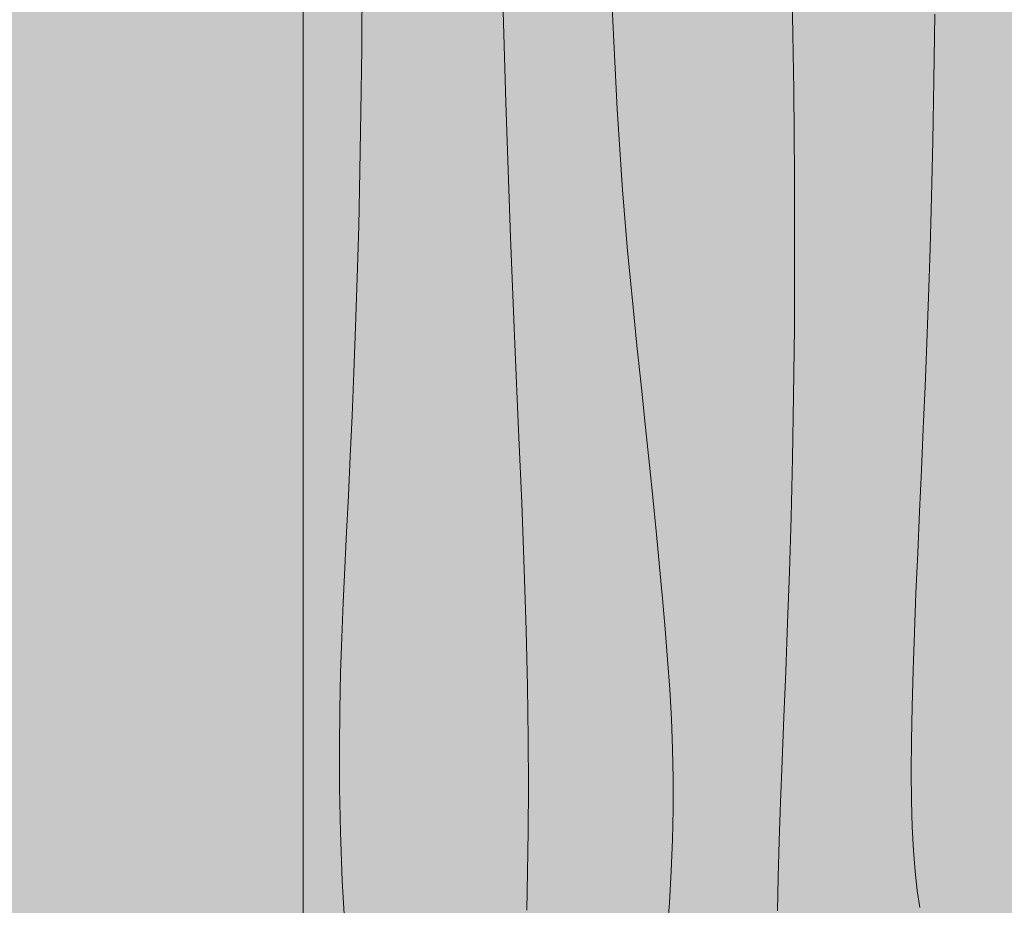
# Model space of a CAD drawing. Units: inches. Extents: x 3024 to 3952, y 1308 to 1863.
# Tile 15 of 29: x 3391.52 to 3411.08, y 1506.34 to 1523.92. Entities that reach past the tile are written whole.
import ezdxf

# ---------------------------------------------------------------- set-up
doc = ezdxf.new("R2010")
doc.units = ezdxf.units.IN
for name, color, linetype, lineweight in [('A-ANNO-DIMS', 2, 'Continuous', 18), ('A-FLOR-TILE-PATT', 7, 'Continuous', 13), ('A-FURN', 8, 'Continuous', 18), ('A-FURN-PATT', 9, 'Continuous', 13)]:
    doc.layers.add(name, color=color, linetype=linetype, lineweight=lineweight)
doc.layers.add('A-FLOR-PATT', color=254, linetype='Continuous', lineweight=13, true_color=0xfeeab9)
doc.styles.get("Standard").update_dxf_attribs({"font": 'arial.ttf'})
doc.dimstyles.get("Standard").update_dxf_attribs({"dimtxt": 0.18, "dimasz": 0.18, "dimexe": 0.18, "dimexo": 0.0625, "dimgap": 0.09, "dimtad": 0, "dimtih": 1, "dimtoh": 1, "dimdec": 4, "dimzin": 0, "dimdsep": 46, "dimtxsty": 'Standard', "dimcen": 0.09, "dimadec": 0, "dimazin": 0, "dimtfac": 1, "dimtdec": 4, "dimtofl": 0, "dimtmove": 0, "dimatfit": 3, "dimfxl": 1, "dimtolj": 1, "dimtzin": 0, "dimarcsym": 0})

# ---------------------------------------------------------------- blocks, each defined once
blk = doc.blocks.new('Table - Rectangular Woodgrain 60 x 30 in.')
blk.add_line((0, -30), (60, -30))
for points in [[(23.6054, -13.2439), (25.3666, -13.2667), (26.9728, -13.2947), (28.4531, -13.3281), (29.8256, -13.3663), (31.1083, -13.4083), (32.3191, -13.4535), (33.476, -13.501), (34.597, -13.5501), (35.7, -13.6), (36.7984, -13.6497), (37.8875, -13.6979), (38.9578, -13.743), (40, -13.7833), (41.0047, -13.8174), (41.9625, -13.8438), (42.864, -13.8607), (43.7, -13.8667), (44.4631, -13.8604), (45.1552, -13.8417), (45.7801, -13.8104), (46.3416, -13.7667), (46.8439, -13.7104), (47.2906, -13.6417)], [(23.1328, -17.0297), (25.6307, -16.9878), (27.9, -16.9667), (29.9928, -16.9617), (31.9302, -16.9703), (33.7254, -16.9907), (35.3917, -17.0208), (36.9423, -17.0588), (38.3906, -17.1026), (39.7499, -17.1503), (41.0333, -17.2), (42.2519, -17.2496), (43.4073, -17.2969), (44.4986, -17.3395), (45.525, -17.375), (46.4858, -17.4012), (47.3802, -17.4156)], [(23.25, -21.8083), (26.1269, -21.6663), (28.2656, -21.5281), (29.884, -21.3947), (31.2, -21.2667), (32.3967, -21.1448), (33.5172, -21.0292), (34.5697, -20.9198), (35.5625, -20.8167), (36.5037, -20.7198), (37.4015, -20.6292), (38.2642, -20.5448), (39.1, -20.4667), (39.9164, -20.3951), (40.7187, -20.3313), (41.5117, -20.2768), (42.3, -20.2333), (43.0883, -20.2024), (43.8812, -20.1854), (44.6836, -20.1841), (45.5, -20.2), (46.3328, -20.234), (47.1747, -20.2844), (48.0163, -20.3488)], [(21.4049, -24.7606), (25.9458, -24.625), (29.529, -24.4988), (32.3578, -24.3844), (34.6359, -24.284), (36.5667, -24.2), (38.3213, -24.1341), (39.9417, -24.0854), (41.437, -24.0523), (42.8167, -24.0333), (44.0901, -24.0268), (45.2667, -24.0313), (46.3557, -24.0451), (47.3667, -24.0667)], [(22.6125, -28.4344), (24.5164, -28.4455), (26.2, -28.4667), (27.762, -28.4947), (29.2276, -28.5281), (30.6033, -28.5663), (31.8958, -28.6084), (33.1118, -28.6535), (34.2578, -28.7011), (35.3405, -28.7501), (36.3666, -28.8), (37.3443, -28.8497), (38.288, -28.8974), (39.2137, -28.9412), (40.1375, -28.9792), (41.0753, -29.0093), (42.0432, -29.0297), (43.0572, -29.0384), (44.1333, -29.0333), (45.2936, -29.0114), (46.5843, -28.9641), (48.0579, -28.8816)]]:
    blk.add_lwpolyline(points)
blk = doc.blocks.new('*D32')
at = {"layer": 'A-ANNO-DIMS', "color": 0, "lineweight": -2, "transparency": 16777216}
for p, q in [((3397.088, 1541.715), (3390.23, 1541.715)), ((3390.41, 1541.535), (3390.41, 1519.428)), ((3390.41, 1496.958), (3390.41, 1519.065)), ((3397.088, 1496.778), (3390.23, 1496.778))]:
    blk.add_line(p, q, dxfattribs=at)
at = {"layer": 'A-ANNO-DIMS', "color": 0, "transparency": 16777216}
for points in [[(3390.38, 1541.535), (3390.44, 1541.535), (3390.41, 1541.715)], [(3390.38, 1496.958), (3390.44, 1496.958), (3390.41, 1496.778)]]:
    blk.add_solid(points, dxfattribs=at)
at = {"layer": 'Defpoints', "color": 0, "transparency": 16777216}
for p in [(3397.15, 1541.715), (3390.41, 1496.778), (3397.15, 1496.778)]:
    blk.add_point(p, dxfattribs=at)
at = {"layer": 'A-ANNO-DIMS', "color": 0, "transparency": 16777216, "insert": (3390.41, 1519.246), "char_height": 0.18, "attachment_point": 5}
blk.add_mtext('\\A1;TABLE 45', dxfattribs=at)
blk = doc.blocks.new('*D104')
at = {"layer": 'A-ANNO-DIMS', "color": 0, "lineweight": -2, "transparency": 16777216}
for p, q in [((3360.648, 1515.787), (3360.828, 1515.787)), ((3360.738, 1515.697), (3360.738, 1515.877)), ((3507.355, 1515.787), (3452.554, 1515.787))]:
    blk.add_line(p, q, dxfattribs=at)
at = {"layer": 'A-ANNO-DIMS', "color": 0, "transparency": 16777216}
blk.add_solid([(3452.554, 1515.817), (3452.554, 1515.757), (3452.374, 1515.787)], dxfattribs=at)
at = {"layer": 'Defpoints', "color": 0, "transparency": 16777216}
for p in [(3360.738, 1515.787), (3452.374, 1515.787)]:
    blk.add_point(p, dxfattribs=at)
at = {"layer": 'A-ANNO-DIMS', "color": 0, "transparency": 16777216, "insert": (3507.835, 1515.787), "char_height": 0.18, "attachment_point": 5}
blk.add_mtext('\\A1;R91.64', dxfattribs=at)
blk = doc.blocks.new('*D105')
at = {"layer": 'A-ANNO-DIMS', "color": 0, "lineweight": -2, "transparency": 16777216}
for p, q in [((3370.437, 1515.787), (3370.617, 1515.787)), ((3370.527, 1515.697), (3370.527, 1515.877)), ((3508.74, 1515.787), (3457.09, 1515.787))]:
    blk.add_line(p, q, dxfattribs=at)
at = {"layer": 'A-ANNO-DIMS', "color": 0, "transparency": 16777216}
blk.add_solid([(3457.09, 1515.817), (3457.09, 1515.757), (3456.91, 1515.787)], dxfattribs=at)
at = {"layer": 'Defpoints', "color": 0, "transparency": 16777216}
for p in [(3370.527, 1515.787), (3456.91, 1515.787)]:
    blk.add_point(p, dxfattribs=at)
at = {"layer": 'A-ANNO-DIMS', "color": 0, "transparency": 16777216, "insert": (3509.22, 1515.787), "char_height": 0.18, "attachment_point": 5}
blk.add_mtext('\\A1;R86.38', dxfattribs=at)

msp = doc.modelspace()

# ---------------------------------------------------------------- hatches: boundary and pattern name
at = {"layer": 'A-FLOR-PATT', "transparency": 33554528}
h = msp.add_hatch(color=256, dxfattribs=at)
h.dxf.hatch_style = 1
h.paths.add_polyline_path([(3460.764, 1688.6064), (3412.764, 1688.6064), (3412.764, 1694.6064), (3460.764, 1694.6064), (3460.764, 1778.6064), (3406.764, 1778.6064), (3406.764, 1759.9514), (3318.2981, 1759.9514), (3318.2981, 1658.6064), (3322.5356, 1658.6064), (3322.5356, 1652.6064), (3292.764, 1652.6064), (3292.764, 1778.6064), (3106.764, 1778.6064), (3106.764, 1628.6064), (3172.764, 1628.6064), (3172.764, 1532.6064), (3166.764, 1532.6064), (3166.764, 1628.6064), (3106.764, 1628.6064), (3106.764, 1356.8452), (3202.812, 1356.8452), (3202.812, 1354.2534), (3202.812, 1353.8388), (3202.812, 1351.1212), (3202.812, 1347.8452), (3277.764, 1347.8452), (3277.764, 1353.8452), (3277.764, 1356.8452), (3277.764, 1442.6064), (3460.764, 1442.6064)])
h.paths.add_polyline_path([(3216.238, 1527.2064), (3216.238, 1491.2064), (3214.663, 1491.2064), (3214.663, 1491.2409, -0.3966224), (3180.243, 1526.6064), (3163.0285, 1526.6064), (3163.0285, 1531.1064), (3161.716, 1531.1064), (3161.716, 1561.1064), (3163.0285, 1561.1064), (3163.0285, 1531.1064), (3163.0285, 1526.6064), (3180.243, 1526.6064, 0.3966224), (3214.663, 1491.2409), (3214.663, 1527.2064)], flags=16)
h.paths.add_polyline_path([(3227.364, 1649.8972), (3191.364, 1649.8972), (3191.364, 1651.4722), (3227.364, 1651.4722)], flags=16)
h.paths.add_polyline_path([(3323.1172, 1606.7362), (3323.8545, 1606.8514), (3323.8545, 1594.8241), (3323.1172, 1594.9393)], flags=16)
h.paths.add_polyline_path([(3324.2232, 1606.909), (3330.1216, 1607.8307), (3330.1216, 1614.1093), (3339.3495, 1614.1093), (3340.2711, 1620.0078), (3352.4136, 1620.0078), (3353.3353, 1614.1093), (3359.9941, 1614.1093), (3360.9157, 1620.0078), (3373.0582, 1620.0078), (3373.9799, 1614.1093), (3383.2077, 1614.1093), (3383.2077, 1607.8307), (3389.1062, 1606.909), (3389.1062, 1594.7665), (3383.2077, 1593.8449), (3383.2077, 1587.5663), (3373.9799, 1587.5663), (3373.0583, 1581.6678), (3360.9157, 1581.6678), (3359.9941, 1587.5663), (3353.3353, 1587.5663), (3352.4136, 1581.6678), (3340.2711, 1581.6678), (3339.3495, 1587.5663), (3330.1216, 1587.5663), (3330.1216, 1593.8449), (3324.2232, 1594.7665)], flags=16)
h.paths.add_polyline_path([(3236.1584, 1693.1064), (3236.1584, 1723.1064), (3237.4709, 1723.1064), (3237.4709, 1693.1064)], flags=16)
h.paths.add_polyline_path([(3373.2158, 1600.6847), (3373.7965, 1600.7303), (3374.3268, 1600.7874), (3374.8132, 1600.8531), (3375.2621, 1600.9247), (3375.6801, 1600.9991), (3376.0736, 1601.0735), (3376.6855, 1601.19), (3377.366, 1601.3023), (3378.0667, 1601.3814), (3378.8026, 1601.4123), (3379.5865, 1601.3839), (3380.4537, 1601.2948), (3381.301, 1601.1717), (3382.0317, 1601.0433), (3382.4398, 1600.9607), (3382.6252, 1600.9201), (3382.919, 1600.8507), (3382.9044, 1600.8531), (3382.842, 1600.8678), (3382.7541, 1600.8896), (3382.6252, 1600.9201), (3382.4398, 1600.9607), (3382.1868, 1601.0119), (3381.8738, 1601.0711), (3381.5125, 1601.1346), (3381.1149, 1601.1988), (3380.6928, 1601.2601), (3380.2581, 1601.3149), (3379.8226, 1601.3597), (3379.3984, 1601.3908), (3378.9944, 1601.4054), (3378.6092, 1601.4042), (3378.2384, 1601.3886), (3377.8777, 1601.36), (3377.5227, 1601.32), (3377.1691, 1601.2698), (3376.8127, 1601.211), (3376.4491, 1601.145), (3376.0736, 1601.0735), (3375.4177, 1600.9494), (3374.5542, 1600.8119), (3373.5044, 1600.6988)], flags=0)
h.paths.add_polyline_path([(3380.0253, 1596.7351), (3380.499, 1596.6659), (3380.9706, 1596.6119), (3381.4375, 1596.5791), (3381.8971, 1596.5736), (3382.5886, 1596.6167), (3382.7848, 1596.6692), (3382.1465, 1596.5706), (3381.236, 1596.5815), (3380.3199, 1596.6865)], flags=0)
h.paths.add_polyline_path([(3369.6414, 1603.9617), (3370.1589, 1604.0021), (3370.6218, 1604.0539), (3371.0335, 1604.1173), (3371.3978, 1604.1921), (3371.7181, 1604.2785), (3371.9984, 1604.3761), (3372.2441, 1604.483), (3372.4611, 1604.5972), (3372.655, 1604.7163), (3372.8317, 1604.8384), (3372.9968, 1604.9611), (3373.3703, 1605.2455), (3373.8426, 1605.5328), (3374.4624, 1605.7539), (3375.1058, 1605.8302), (3375.7221, 1605.8261), (3376.4109, 1605.76), (3377.1534, 1605.6376), (3377.8945, 1605.473), (3378.1382, 1605.409), (3377.7394, 1605.5074), (3377.3509, 1605.5937), (3376.9704, 1605.6677), (3376.5999, 1605.7288), (3376.2417, 1605.7762), (3375.8979, 1605.8092), (3375.5707, 1605.8271), (3375.2621, 1605.8291), (3374.9745, 1605.8146), (3374.7092, 1605.7832), (3374.4647, 1605.7359), (3374.239, 1605.6742), (3374.0298, 1605.5996), (3373.835, 1605.5134), (3373.6525, 1605.4171), (3373.4801, 1605.3123), (3373.3156, 1605.2002), (3373.1562, 1605.0825), (3372.7603, 1604.781), (3372.236, 1604.4588), (3371.5738, 1604.2283), (3370.8493, 1604.0794), (3369.9262, 1603.976)], flags=0)
h.paths.add_polyline_path([(3366.7533, 1606.5832), (3367.1713, 1606.5519), (3367.5378, 1606.5374), (3367.8568, 1606.5394), (3368.1325, 1606.5573), (3368.3694, 1606.5903), (3368.5717, 1606.6377), (3368.7438, 1606.6988), (3368.89, 1606.7728), (3369.0146, 1606.8591), (3369.121, 1606.9568), (3369.2094, 1607.0646), (3369.2792, 1607.181), (3369.3295, 1607.3046), (3369.3596, 1607.4339), (3369.3688, 1607.5676), (3369.3565, 1607.7042), (3369.3218, 1607.8422), (3369.2649, 1607.9804), (3369.1893, 1608.1187), (3369.0993, 1608.2569), (3368.9992, 1608.3952), (3368.8934, 1608.5334), (3368.7861, 1608.6717), (3368.6817, 1608.8099), (3368.4212, 1609.1804), (3368.2685, 1609.7106), (3368.4883, 1610.1814), (3369.0537, 1610.4604), (3369.6717, 1610.5097), (3370.2812, 1610.3612), (3370.4805, 1610.2968), (3370.1882, 1610.3839), (3369.9284, 1610.4472), (3369.6905, 1610.4842), (3369.4662, 1610.4933), (3369.2555, 1610.4765), (3369.0608, 1610.4367), (3368.884, 1610.3767), (3368.7274, 1610.2994), (3368.5931, 1610.2077), (3368.4833, 1610.1045), (3368.4002, 1609.9927), (3368.3451, 1609.8747), (3368.3166, 1609.7517), (3368.3127, 1609.6244), (3368.331, 1609.4935), (3368.3696, 1609.3597), (3368.4261, 1609.2237), (3368.4985, 1609.0863), (3368.5845, 1608.9482), (3368.6817, 1608.8099), (3368.7861, 1608.6717), (3368.8934, 1608.5334), (3368.9992, 1608.3952), (3369.0993, 1608.2569), (3369.3398, 1607.8876), (3369.3941, 1607.2896), (3368.9774, 1606.7817), (3368.3928, 1606.5742), (3367.7162, 1606.5303), (3367.0044, 1606.5585)], flags=0)
h.paths.add_polyline_path([(3362.1859, 1610.2589), (3362.5478, 1610.2845), (3362.8348, 1610.3275), (3363.0585, 1610.3863), (3363.2303, 1610.4595), (3363.3619, 1610.5457), (3363.463, 1610.6432), (3363.5376, 1610.7502), (3363.5876, 1610.8643), (3363.6153, 1610.9834), (3363.6229, 1611.1055), (3363.6125, 1611.2283), (3363.5861, 1611.3496), (3363.5462, 1611.4673), (3363.4949, 1611.5797), (3363.4358, 1611.6871), (3363.3723, 1611.7902), (3363.3081, 1611.8897), (3363.2468, 1611.9863), (3363.192, 1612.0808), (3363.0258, 1612.4261), (3363.3371, 1612.8672), (3363.9008, 1612.9782), (3364.4822, 1612.9641), (3365.1098, 1612.9074), (3365.328, 1612.8805), (3364.9615, 1612.9208), (3364.6426, 1612.9496), (3364.3668, 1612.9669), (3364.1299, 1612.9726), (3363.9276, 1612.9669), (3363.7555, 1612.9496), (3363.6093, 1612.9208), (3363.4848, 1612.8805), (3363.3782, 1612.8289), (3363.2889, 1612.7672), (3363.2169, 1612.6969), (3363.1622, 1612.6193), (3363.1247, 1612.5361), (3363.1046, 1612.4484), (3363.1017, 1612.358), (3363.1161, 1612.266), (3363.1472, 1612.1738), (3363.192, 1612.0808), (3363.2468, 1611.9863), (3363.3081, 1611.8897), (3363.3723, 1611.7902), (3363.4358, 1611.6871), (3363.6363, 1611.323), (3363.5979, 1610.7003), (3363.0863, 1610.3651), (3362.3983, 1610.2622)], flags=0)
h.paths.add_polyline_path([(3352.356, 1581.2991), (3352.2408, 1580.5618), (3340.4439, 1580.5618), (3340.3287, 1581.2991)], flags=16)
h.paths.add_polyline_path([(3340.4439, 1621.1137), (3352.2408, 1621.1137), (3352.356, 1620.3764), (3340.3287, 1620.3764)], flags=16)
h.paths.add_polyline_path([(3278.4282, 1504.7424), (3290.3831, 1504.7424), (3290.3831, 1502.7499), (3291.0473, 1502.7499), (3291.0473, 1494.7799), (3290.3831, 1494.7799), (3290.3831, 1494.1158), (3291.0473, 1494.1158), (3291.0473, 1486.1458), (3290.3831, 1486.1458), (3290.3831, 1484.1533), (3291.0473, 1484.1533), (3291.0473, 1483.4892, -0.0909091), (3291.0473, 1468.8776), (3291.0473, 1468.2135), (3290.3831, 1468.2135), (3290.3831, 1464.8926), (3278.4282, 1464.8926), (3278.4282, 1472.8626), (3277.764, 1473.5268), (3277.764, 1478.84), (3278.4282, 1479.5042)], flags=16)
h.paths.add_polyline_path([(3278.7603, 1504.4103), (3290.051, 1504.4103), (3290.051, 1465.2247), (3278.7603, 1465.2247)], flags=0)
h.paths.add_polyline_path([(3123.904, 1600.7821), (3117.9039, 1602.7821), (3117.9039, 1599.7821), (3119.4039, 1599.7821), (3119.4039, 1596.7821), (3118.4039, 1596.7821), (3118.4039, 1598.7821), (3117.9039, 1598.7821), (3117.9039, 1596.2821), (3109.9039, 1596.2821), (3109.9039, 1617.2821), (3117.9039, 1617.2821), (3117.9039, 1610.7821), (3123.9038, 1612.7821, -0.7025712), (3137.9039, 1606.7822, -0.7025621)], flags=16)
h.paths.add_polyline_path([(3123.9039, 1602.7822), (3123.9039, 1610.7822, -0.7345333), (3136.9039, 1606.7822, -0.7345297)], flags=0)
h.paths.add_polyline_path([(3177.972, 1689.6473), (3109.2405, 1689.6473), (3109.2405, 1741.1959), (3177.972, 1741.1959)], flags=16)
h.paths.add_polyline_path([(3373.0006, 1581.2991), (3372.8854, 1580.5618), (3361.0885, 1580.5618), (3360.9733, 1581.2991)], flags=16)
h.paths.add_polyline_path([(3361.0885, 1621.1137), (3372.8854, 1621.1137), (3373.0006, 1620.3764), (3360.9733, 1620.3764)], flags=16)
h.paths.add_polyline_path([(3116.9039, 1598.2821, -0.4142136), (3116.1539, 1597.2821), (3111.9039, 1597.2821, -0.4142136), (3110.9039, 1598.0321), (3110.9039, 1615.2821, -0.4142136), (3111.6539, 1616.2821), (3115.9039, 1616.2821, -0.4142136), (3116.9039, 1615.5321)], flags=0)
h.paths.add_polyline_path([(3121.6122, 1728.1369), (3121.6122, 1696.5205), (3110.2715, 1696.5205), (3110.2715, 1714.3906), (3121.6122, 1714.3906), (3121.6122, 1716.4526), (3110.2715, 1716.4526), (3110.2715, 1734.3228), (3123.3304, 1734.3228), (3123.3304, 1729.8552), (3134.6711, 1741.1959), (3134.6711, 1728.1369)], flags=0)
h.paths.add_polyline_path([(3389.4748, 1606.8514), (3390.2122, 1606.7362), (3390.2122, 1594.9393), (3389.4748, 1594.8241)], flags=16)
h.paths.add_polyline_path([(3257.6842, 1762.8281), (3259.6842, 1768.8281), (3256.6842, 1768.8281), (3256.6842, 1767.3281), (3253.6842, 1767.3281), (3253.6842, 1768.3281), (3255.6842, 1768.3281), (3255.6842, 1768.8281), (3253.1842, 1768.8281), (3253.1842, 1776.8281), (3274.1842, 1776.8281), (3274.1842, 1768.8281), (3267.6842, 1768.8281), (3269.6842, 1762.8282, -0.7025712), (3263.6843, 1748.8282, -0.7025621)], flags=16)
h.paths.add_polyline_path([(3259.6842, 1762.8281), (3267.6843, 1762.8281, -0.7345333), (3263.6842, 1749.8282, -0.7345297)], flags=0)
h.paths.add_polyline_path([(3411.264, 1715.6064), (3411.264, 1716.9189), (3441.264, 1716.9189), (3441.264, 1715.6064)], flags=16)
h.paths.add_polyline_path([(3178.3806, 1449.1876), (3178.3806, 1397.639), (3109.6491, 1397.639), (3109.6491, 1449.1876)], flags=16)
h.paths.add_polyline_path([(3397.1501, 1541.7146), (3419.6183, 1541.7146), (3419.6183, 1496.7783), (3397.1501, 1496.7783)], flags=16)
h.paths.add_polyline_path([(3254.1842, 1770.5781), (3254.1842, 1774.8281, -0.4142136), (3254.9342, 1775.8281), (3272.1842, 1775.8281, -0.4142136), (3273.1842, 1775.0781), (3273.1842, 1770.8281, -0.4142136), (3272.4342, 1769.8281), (3255.1842, 1769.8281, -0.4142136)], flags=0)
h.paths.add_polyline_path([(3403.672, 1500.7601), (3403.6016, 1500.3997), (3403.5328, 1500.0441), (3403.4662, 1499.6867), (3403.4027, 1499.3226), (3403.3464, 1498.9532), (3403.3025, 1498.5811), (3403.2759, 1498.2091), (3403.2714, 1497.8401), (3403.3064, 1497.2813), (3403.3491, 1497.1219), (3403.2689, 1497.6395), (3403.2778, 1498.3719), (3403.3635, 1499.0984), (3403.4889, 1499.8168), (3403.6016, 1500.3997), (3403.672, 1500.7601), (3403.744, 1501.1315), (3403.817, 1501.5205), (3403.891, 1501.9336), (3403.9656, 1502.3769), (3404.0404, 1502.8572), (3404.115, 1503.3786), (3404.2264, 1504.2311), (3404.2571, 1504.5223), (3404.1552, 1503.6598), (3404.0063, 1502.6193), (3403.8604, 1501.7518), (3403.744, 1501.1315)], flags=0)
h.paths.add_polyline_path([(3406.5868, 1505.0416), (3406.6121, 1504.5236), (3406.6492, 1504.0526), (3406.6956, 1503.624), (3406.7491, 1503.2333), (3406.8072, 1502.8759), (3406.8676, 1502.5473), (3406.9281, 1502.243), (3407.0268, 1501.7597), (3407.1416, 1501.1368), (3407.2087, 1500.3904), (3407.1804, 1499.6703), (3407.1078, 1498.9956), (3407.0074, 1498.3199), (3406.8809, 1497.6059), (3406.7403, 1496.9627), (3406.7418, 1496.9824), (3406.7491, 1497.0249), (3406.8229, 1497.3409), (3406.8364, 1497.4025), (3406.878, 1497.6078), (3406.9261, 1497.8614), (3406.9777, 1498.1526), (3407.0298, 1498.4712), (3407.0797, 1498.8068), (3407.1243, 1499.149), (3407.1607, 1499.4874), (3407.1859, 1499.8115), (3407.1978, 1500.1137), (3407.1969, 1500.3962), (3407.1841, 1500.6642), (3407.1609, 1500.9225), (3407.1284, 1501.1761), (3407.0876, 1501.43), (3407.0398, 1501.6891), (3406.9862, 1501.9585), (3406.8832, 1502.4628), (3406.7712, 1503.0713), (3406.6657, 1503.8424), (3406.5924, 1504.7735)], flags=0)
h.paths.add_polyline_path([(3409.2517, 1507.8962), (3409.2752, 1507.4282), (3409.3079, 1507.0076), (3409.3501, 1506.6314), (3409.4015, 1506.2969), (3409.4624, 1506.0009), (3409.5326, 1505.7406), (3409.6119, 1505.5128), (3409.6988, 1505.3131), (3409.7915, 1505.1368), (3409.8883, 1504.9792), (3409.9875, 1504.8356), (3410.0872, 1504.7015), (3410.1859, 1504.572), (3410.4508, 1504.2132), (3410.7205, 1503.6035), (3410.8059, 1502.8824), (3410.7619, 1502.0875), (3410.6122, 1501.2299), (3410.4402, 1500.6169), (3410.2538, 1500.0031), (3410.0536, 1499.3219), (3409.9909, 1499.0812), (3410.1761, 1499.7472), (3410.3596, 1500.3513), (3410.4512, 1500.6561), (3410.5312, 1500.9412), (3410.6013, 1501.226), (3410.6614, 1501.512), (3410.7111, 1501.7964), (3410.7496, 1502.0763), (3410.7764, 1502.3489), (3410.7909, 1502.6114), (3410.7926, 1502.8608), (3410.7808, 1503.0944), (3410.7553, 1503.31), (3410.7169, 1503.5087), (3410.6667, 1503.6921), (3410.6061, 1503.8621), (3410.5361, 1504.0203), (3410.4578, 1504.1686), (3410.3726, 1504.3088), (3410.2815, 1504.4424), (3410.1859, 1504.572), (3410.0872, 1504.7015), (3409.859, 1505.0083), (3409.5943, 1505.5117), (3409.4266, 1506.1336), (3409.324, 1506.8011), (3409.2586, 1507.6407)], flags=0)
h.paths.add_polyline_path([(3411.4914, 1510.5878), (3411.4432, 1510.1586), (3411.4054, 1509.775), (3411.38, 1509.4354), (3411.3681, 1509.1376), (3411.3698, 1508.8784), (3411.3843, 1508.6542), (3411.4112, 1508.4618), (3411.4497, 1508.2974), (3411.4994, 1508.1575), (3411.5595, 1508.0388), (3411.6296, 1507.9375), (3411.7097, 1507.851), (3411.802, 1507.7792), (3411.9096, 1507.7225), (3412.0353, 1507.6817), (3412.1821, 1507.6572), (3412.3528, 1507.6496), (3412.5505, 1507.6597), (3412.778, 1507.6879), (3413.0364, 1507.7341), (3413.3194, 1507.7955), (3413.6188, 1507.8687), (3413.9264, 1507.95), (3414.234, 1508.036), (3414.5333, 1508.1232), (3414.8163, 1508.208), (3415.0747, 1508.287), (3415.3023, 1508.3569), (3415.5007, 1508.4158), (3415.6733, 1508.4617), (3416.1158, 1508.5538), (3416.512, 1508.2591), (3416.716, 1507.6581), (3416.61, 1507.0003), (3416.3052, 1506.3411), (3415.8928, 1505.618), (3415.7339, 1505.3633), (3415.9914, 1505.791), (3416.201, 1506.1583), (3416.3666, 1506.4739), (3416.4925, 1506.7462), (3416.5828, 1506.9838), (3416.6413, 1507.1949), (3416.6725, 1507.3883), (3416.6799, 1507.5705), (3416.6662, 1507.7417), (3416.6339, 1507.9), (3416.5851, 1508.0436), (3416.5223, 1508.1709), (3416.4478, 1508.28), (3416.3639, 1508.3692), (3416.273, 1508.4368), (3416.1765, 1508.4815), (3416.0718, 1508.5047), (3415.9553, 1508.5079), (3415.8237, 1508.493), (3415.6733, 1508.4617), (3415.5007, 1508.4158), (3415.3327, 1508.3659), (3414.6495, 1508.157), (3414.0606, 1507.9855), (3413.4456, 1507.8229), (3412.8838, 1507.701), (3412.5505, 1507.6597), (3412.0748, 1507.6354), (3411.595, 1507.8883), (3411.398, 1508.4429), (3411.3624, 1508.9927), (3411.3854, 1509.5711), (3411.4578, 1510.3071)], flags=0)
h.paths.add_polyline_path([(3135.0797, 1449.1876), (3135.0797, 1436.1286), (3122.0208, 1436.1286), (3122.0208, 1404.5122), (3110.6801, 1404.5122), (3110.6801, 1422.3823), (3122.0208, 1422.3823), (3122.0208, 1424.4443), (3110.6801, 1424.4443), (3110.6801, 1442.3145), (3123.739, 1442.3145), (3123.739, 1437.8469)], flags=0)
h.paths.add_polyline_path([(3416.4944, 1514.2949), (3416.4837, 1513.8511), (3416.4893, 1513.4867), (3416.5102, 1513.1926), (3416.5451, 1512.9593), (3416.5929, 1512.7775), (3416.6524, 1512.6379), (3416.7224, 1512.531), (3416.8017, 1512.4488), (3416.8886, 1512.3882), (3416.9813, 1512.3476), (3417.0781, 1512.3251), (3417.1773, 1512.3189), (3417.277, 1512.3274), (3417.3757, 1512.3488), (3417.4713, 1512.3813), (3417.5627, 1512.4229), (3417.65, 1512.471), (3417.7338, 1512.5225), (3417.8146, 1512.5747), (3417.8931, 1512.6245), (3417.9699, 1512.6691), (3418.2968, 1512.8265), (3418.6505, 1512.4645), (3418.7037, 1511.9342), (3418.6693, 1511.3839), (3418.6076, 1510.8228), (3418.5777, 1510.5927), (3418.6197, 1510.9333), (3418.6525, 1511.2311), (3418.6759, 1511.4903), (3418.6899, 1511.7144), (3418.6946, 1511.9069), (3418.6899, 1512.0713), (3418.6759, 1512.2112), (3418.6525, 1512.33), (3418.6197, 1512.4311), (3418.5778, 1512.5177), (3418.5276, 1512.5903), (3418.4705, 1512.6488), (3418.4075, 1512.6933), (3418.3399, 1512.7237), (3418.2686, 1512.7401), (3418.1951, 1512.7424), (3418.1204, 1512.7307), (3418.0455, 1512.7055), (3417.9792, 1512.6736), (3417.65, 1512.471), (3417.5627, 1512.4229), (3417.4713, 1512.3813), (3417.3757, 1512.3488), (3417.277, 1512.3274), (3416.878, 1512.2936), (3416.5757, 1512.7549), (3416.492, 1513.3145), (3416.4808, 1514.0384)], flags=0)
h.paths.add_polyline_path([(3392.8223, 1481.9454), (3396.7707, 1481.9454), (3396.7707, 1480.9201), (3428.3585, 1480.9201), (3428.3585, 1481.9454), (3432.3069, 1481.9454), (3432.3069, 1464.8354, -0.266667), (3392.8223, 1464.8354)], flags=16)
h.paths.add_polyline_path([(3431.203, 1547.5428), (3450.8613, 1547.5428, -0.1904762), (3450.8614, 1484.031), (3431.203, 1484.031), (3431.203, 1488.5675), (3432.3809, 1488.5675), (3432.3809, 1543.0062), (3431.203, 1543.0062)], flags=16)
h.paths.add_polyline_path([(3451.9233, 1524.86, -0.0496282), (3451.9233, 1506.7138), (3446.7921, 1506.7138), (3446.7921, 1524.86)], flags=0)
h.paths.add_polyline_path([(3460.764, 1436.6064), (3277.764, 1436.6064), (3277.764, 1356.8452), (3277.764, 1353.8452), (3460.764, 1353.8452)], flags=17)
h.paths.add_polyline_path([(3121.3033, 1577.378), (3153.693, 1577.378), (3153.693, 1586.6752), (3121.3033, 1586.6752)], flags=24)
h.paths.add_polyline_path([(3164.1457, 1464.1276), (3210.4801, 1464.1276), (3210.4801, 1473.4247), (3164.1457, 1473.4247)], flags=24)
h.paths.add_polyline_path([(3343.1909, 1505.8863), (3373.7236, 1505.8863), (3373.7236, 1515.1773), (3343.1909, 1515.1773)], flags=24)
h.paths.add_polyline_path([(3337.6353, 1564.2926), (3370.0189, 1564.2926), (3370.0189, 1573.5836), (3337.6353, 1573.5836)], flags=24)
h.paths.add_polyline_path([(3419.204, 1753.8578), (3453.3997, 1753.8578), (3453.3997, 1762.9956), (3419.204, 1762.9956)], flags=24)
h.paths.add_polyline_path([(3341.2523, 1701.0246), (3381.0761, 1701.0246), (3381.0761, 1710.3156), (3341.2523, 1710.3156)], flags=24)
h.paths.add_polyline_path([(3245.8895, 1726.2997), (3278.2793, 1726.2997), (3278.2793, 1735.5968), (3245.8895, 1735.5968)], flags=24)
h.paths.add_polyline_path([(3128.8045, 1668.6736), (3175.1389, 1668.6736), (3175.1389, 1677.9707), (3128.8045, 1677.9707)], flags=24)
h.paths.add_polyline_path([(3345.9997, 1396.0062), (3389.09, 1396.0062), (3389.09, 1405.3033), (3345.9997, 1405.3033)], flags=24)
at = {"layer": 'A-FLOR-TILE-PATT', "transparency": 33554569}
h = msp.add_hatch(dxfattribs=at)
h.set_pattern_fill('ANGLE', color=256, scale=2)
h.set_pattern_definition([(0, (0, 0), (0, 13.97), [10.16, -3.81]), (90, (0, 0), (-13.97, 9e-16), [10.16, -3.81])])
h.paths.add_polyline_path([(3292.764, 1778.6064), (3232.764, 1778.6064), (3232.764, 1694.6064), (3236.1584, 1694.6064), (3236.1584, 1723.1064), (3237.4709, 1723.1064), (3237.4709, 1723.0777, -0.3870039), (3266.1209, 1694.6064), (3292.764, 1694.6064)])
h.paths.add_polyline_path([(3263.6843, 1748.8282, -0.7025621), (3257.6842, 1762.8281), (3259.6842, 1768.8281), (3256.6842, 1768.8281), (3256.6842, 1767.3281), (3253.6842, 1767.3281), (3253.6842, 1768.3281), (3255.6842, 1768.3281), (3255.6842, 1768.8281), (3253.1842, 1768.8281), (3253.1842, 1776.8281), (3274.1842, 1776.8281), (3274.1842, 1768.8281), (3267.6842, 1768.8281), (3269.6842, 1762.8282, -0.7025712)], flags=16)
h.paths.add_polyline_path([(3263.6842, 1749.8282, -0.7345297), (3259.6842, 1762.8281), (3267.6843, 1762.8281, -0.7345333)], flags=0)
h.paths.add_polyline_path([(3255.1842, 1769.8281, -0.4142136), (3254.1842, 1770.5781), (3254.1842, 1774.8281, -0.4142136), (3254.9342, 1775.8281), (3272.1842, 1775.8281, -0.4142136), (3273.1842, 1775.0781), (3273.1842, 1770.8281, -0.4142136), (3272.4342, 1769.8281)], flags=0)
h.paths.add_polyline_path([(3460.764, 1436.6064), (3277.764, 1436.6064), (3277.764, 1356.8452), (3277.764, 1353.8452), (3460.764, 1353.8452)])
h.paths.add_polyline_path([(3166.764, 1628.6064), (3106.764, 1628.6064), (3106.764, 1532.6064), (3133.066, 1532.6064, -0.3870039), (3161.716, 1561.0777), (3161.716, 1561.1064), (3163.0285, 1561.1064), (3163.0285, 1532.6064), (3166.764, 1532.6064)])
h.paths.add_polyline_path([(3123.904, 1600.7821), (3117.9039, 1602.7821), (3117.9039, 1599.7821), (3119.4039, 1599.7821), (3119.4039, 1596.7821), (3118.4039, 1596.7821), (3118.4039, 1598.7821), (3117.9039, 1598.7821), (3117.9039, 1596.2821), (3109.9039, 1596.2821), (3109.9039, 1617.2821), (3117.9039, 1617.2821), (3117.9039, 1610.7821), (3123.9038, 1612.7821, -0.7025712), (3137.9039, 1606.7822, -0.7025621)], flags=16)
h.paths.add_polyline_path([(3123.9039, 1602.7822), (3123.9039, 1610.7822, -0.7345333), (3136.9039, 1606.7822, -0.7345297)], flags=0)
h.paths.add_polyline_path([(3116.1539, 1597.2821), (3111.9039, 1597.2821, -0.4142136), (3110.9039, 1598.0321), (3110.9039, 1615.2821, -0.4142136), (3111.6539, 1616.2821), (3115.9039, 1616.2821, -0.4142136), (3116.9039, 1615.5321), (3116.9039, 1598.2821, -0.4142136)], flags=0)
h.paths.add_polyline_path([(3245.8895, 1726.2997), (3278.2793, 1726.2997), (3278.2793, 1735.5968), (3245.8895, 1735.5968)], flags=24)
h.paths.add_polyline_path([(3345.9997, 1396.0062), (3389.09, 1396.0062), (3389.09, 1405.3033), (3345.9997, 1405.3033)], flags=24)
h.paths.add_polyline_path([(3121.3033, 1577.378), (3153.693, 1577.378), (3153.693, 1586.6752), (3121.3033, 1586.6752)], flags=24)
at = {"layer": 'A-FURN-PATT', "transparency": 33554600}
h = msp.add_hatch(color=256, dxfattribs=at)
h.dxf.hatch_style = 1
h.paths.add_polyline_path([(3417.3334, 1524.2182), (3417.4417, 1525.8535), (3417.5429, 1527.6959), (3417.6336, 1529.794), (3417.7102, 1532.1964), (3417.7693, 1534.9516), (3417.8074, 1538.1081), (3417.8209, 1541.7146), (3412.7281, 1541.7146), (3412.8136, 1536.7897), (3412.8505, 1532.7734), (3412.8466, 1529.5424), (3412.8092, 1526.9731), (3412.7461, 1524.942), (3412.6649, 1523.3259), (3412.5731, 1522.0011), (3412.4784, 1520.8443), (3412.3871, 1519.7527), (3412.2998, 1518.707), (3412.216, 1517.7088), (3412.1351, 1516.7594), (3412.0566, 1515.8603), (3411.9799, 1515.013), (3411.9043, 1514.219), (3411.8293, 1513.4797), (3411.7548, 1512.7959), (3411.6819, 1512.1667), (3411.6125, 1511.5901), (3411.5485, 1511.0643), (3411.4914, 1510.5878), (3411.4432, 1510.1586), (3411.4054, 1509.775), (3411.38, 1509.4354), (3411.3681, 1509.1376), (3411.3698, 1508.8784), (3411.3843, 1508.6542), (3411.4112, 1508.4618), (3411.4497, 1508.2974), (3411.4994, 1508.1575), (3411.5595, 1508.0388), (3411.6296, 1507.9375), (3411.7097, 1507.851), (3411.802, 1507.7792), (3411.9096, 1507.7225), (3412.0353, 1507.6817), (3412.1821, 1507.6572), (3412.3528, 1507.6496), (3412.5505, 1507.6597), (3412.778, 1507.6879), (3413.0364, 1507.7341), (3413.3194, 1507.7955), (3413.6188, 1507.8687), (3413.9264, 1507.95), (3414.234, 1508.036), (3414.5333, 1508.1232), (3414.8163, 1508.208), (3415.0747, 1508.287), (3415.4508, 1508.4025), (3415.8572, 1508.5106), (3416.186, 1508.5015), (3416.4107, 1508.3344), (3416.5614, 1508.1136), (3416.6596, 1507.8241), (3416.6872, 1507.4795), (3416.6413, 1507.1949), (3416.5828, 1506.9838), (3416.4925, 1506.7462), (3416.3666, 1506.4739), (3416.201, 1506.1583), (3415.9914, 1505.791), (3415.7339, 1505.3633), (3415.4242, 1504.8669), (3415.0615, 1504.292), (3414.6566, 1503.6241), (3414.2236, 1502.8473), (3413.7766, 1501.946), (3413.3295, 1500.9042), (3412.8966, 1499.7062), (3412.4917, 1498.3362), (3412.1289, 1496.7783), (3417.2217, 1496.7783), (3417.334, 1498.1918), (3417.4456, 1499.5619), (3417.5561, 1500.8806), (3417.6648, 1502.1395), (3417.7712, 1503.3306), (3417.8747, 1504.4456), (3417.9746, 1505.4763), (3418.0705, 1506.4147), (3418.1617, 1507.2549), (3418.2476, 1508.0019), (3418.3277, 1508.6628), (3418.4013, 1509.245), (3418.4679, 1509.7559), (3418.5269, 1510.2027), (3418.5777, 1510.5927), (3418.6197, 1510.9333), (3418.6525, 1511.2311), (3418.6759, 1511.4903), (3418.6899, 1511.7144), (3418.6946, 1511.9069), (3418.6899, 1512.0713), (3418.6759, 1512.2112), (3418.6525, 1512.33), (3418.6197, 1512.4311), (3418.5778, 1512.5177), (3418.5276, 1512.5903), (3418.4705, 1512.6488), (3418.4075, 1512.6933), (3418.3399, 1512.7237), (3418.2686, 1512.7401), (3418.1951, 1512.7424), (3418.1204, 1512.7307), (3418.0455, 1512.7055), (3417.9699, 1512.6691), (3417.8931, 1512.6245), (3417.8146, 1512.5747), (3417.5633, 1512.4125), (3417.2709, 1512.3131), (3416.9695, 1512.3318), (3416.7549, 1512.4815), (3416.6143, 1512.696), (3416.5451, 1512.9593), (3416.5102, 1513.1926), (3416.4893, 1513.4867), (3416.4837, 1513.8511), (3416.4944, 1514.2949), (3416.5226, 1514.8277), (3416.5691, 1515.4576), (3416.6319, 1516.1871), (3416.7088, 1517.0179), (3416.7973, 1517.9515), (3416.8952, 1518.9891), (3417.0002, 1520.1323), (3417.1097, 1521.3827), (3417.2217, 1522.7416)])
h.paths.add_polyline_path([(3419.6183, 1541.7146), (3417.8209, 1541.7146), (3417.8074, 1538.1081), (3417.7693, 1534.9516), (3417.7102, 1532.1964), (3417.6336, 1529.794), (3417.5429, 1527.6959), (3417.4417, 1525.8535), (3417.3334, 1524.2182), (3417.2217, 1522.7416), (3417.1097, 1521.3827), (3417.0002, 1520.1323), (3416.8952, 1518.9891), (3416.7973, 1517.9515), (3416.7088, 1517.0179), (3416.6319, 1516.1871), (3416.5691, 1515.4576), (3416.5226, 1514.8277), (3416.4944, 1514.2949), (3416.4837, 1513.8511), (3416.4893, 1513.4867), (3416.5102, 1513.1926), (3416.5451, 1512.9593), (3416.5929, 1512.7775), (3416.6524, 1512.6379), (3416.7224, 1512.531), (3416.8017, 1512.4488), (3416.8886, 1512.3882), (3416.9813, 1512.3476), (3417.0781, 1512.3251), (3417.1773, 1512.3189), (3417.277, 1512.3274), (3417.3757, 1512.3488), (3417.4713, 1512.3813), (3417.5627, 1512.4229), (3417.65, 1512.471), (3417.7338, 1512.5225), (3417.9865, 1512.6856), (3418.237, 1512.7699), (3418.4785, 1512.6613), (3418.6304, 1512.4416), (3418.6876, 1512.1519), (3418.6969, 1511.8267), (3418.6759, 1511.4903), (3418.6525, 1511.2311), (3418.6197, 1510.9333), (3418.5777, 1510.5927), (3418.5269, 1510.2027), (3418.4679, 1509.7559), (3418.4013, 1509.245), (3418.3277, 1508.6628), (3418.2476, 1508.0019), (3418.1617, 1507.2549), (3418.0705, 1506.4147), (3417.9746, 1505.4763), (3417.8747, 1504.4456), (3417.7712, 1503.3306), (3417.6648, 1502.1395), (3417.5561, 1500.8806), (3417.4456, 1499.5619), (3417.334, 1498.1918), (3417.2217, 1496.7783), (3419.6183, 1496.7783)])
h.paths.add_polyline_path([(3412.5731, 1522.0011), (3412.6649, 1523.3259), (3412.7461, 1524.942), (3412.8092, 1526.9731), (3412.8466, 1529.5424), (3412.8505, 1532.7734), (3412.8136, 1536.7897), (3412.7281, 1541.7146), (3410.0319, 1541.7146), (3409.9329, 1537.8316), (3409.8579, 1534.5089), (3409.8028, 1531.6816), (3409.7635, 1529.2854), (3409.7359, 1527.2554), (3409.7159, 1525.5271), (3409.6994, 1524.0356), (3409.6824, 1522.7166), (3409.6614, 1521.5137), (3409.6364, 1520.405), (3409.6078, 1519.3771), (3409.5763, 1518.4164), (3409.5425, 1517.5096), (3409.5069, 1516.6432), (3409.4701, 1515.8036), (3409.4327, 1514.9775), (3409.3955, 1514.1549), (3409.3594, 1513.3392), (3409.3256, 1512.5376), (3409.2955, 1511.7571), (3409.2699, 1511.0046), (3409.2501, 1510.2873), (3409.2375, 1509.6121), (3409.233, 1508.986), (3409.2377, 1508.4145), (3409.2517, 1507.8962), (3409.2752, 1507.4282), (3409.3079, 1507.0076), (3409.3501, 1506.6314), (3409.4015, 1506.2969), (3409.4624, 1506.0009), (3409.5326, 1505.7406), (3409.6119, 1505.5128), (3409.6988, 1505.3131), (3409.7915, 1505.1368), (3409.8883, 1504.9792), (3409.9875, 1504.8356), (3410.0872, 1504.7015), (3410.3178, 1504.3987), (3410.5042, 1504.0923), (3410.643, 1503.7787), (3410.7431, 1503.4127), (3410.7808, 1503.0944), (3410.7926, 1502.8608), (3410.7909, 1502.6114), (3410.7764, 1502.3489), (3410.7496, 1502.0763), (3410.7111, 1501.7964), (3410.6614, 1501.512), (3410.6013, 1501.226), (3410.5312, 1500.9412), (3410.4512, 1500.6561), (3410.3596, 1500.3513), (3410.2538, 1500.0031), (3410.1317, 1499.5877), (3409.9909, 1499.0812), (3409.8291, 1498.4601), (3409.6438, 1497.7003), (3409.4327, 1496.7783), (3412.1289, 1496.7783), (3412.4917, 1498.3362), (3412.8966, 1499.7062), (3413.3295, 1500.9042), (3413.7766, 1501.946), (3414.2236, 1502.8473), (3414.6566, 1503.6241), (3415.0615, 1504.292), (3415.4242, 1504.8669), (3415.7339, 1505.3633), (3415.9914, 1505.791), (3416.201, 1506.1583), (3416.3666, 1506.4739), (3416.4925, 1506.7462), (3416.5828, 1506.9838), (3416.6413, 1507.1949), (3416.6725, 1507.3883), (3416.6799, 1507.5705), (3416.6662, 1507.7417), (3416.6339, 1507.9), (3416.5851, 1508.0436), (3416.5223, 1508.1709), (3416.4478, 1508.28), (3416.3639, 1508.3692), (3416.273, 1508.4368), (3416.1765, 1508.4815), (3416.0718, 1508.5047), (3415.9553, 1508.5079), (3415.8237, 1508.493), (3415.6733, 1508.4617), (3415.5007, 1508.4158), (3415.3023, 1508.3569), (3414.8599, 1508.2211), (3414.5333, 1508.1232), (3414.234, 1508.036), (3413.9264, 1507.95), (3413.6188, 1507.8687), (3413.3194, 1507.7955), (3412.8838, 1507.701), (3412.4382, 1507.6458), (3412.0995, 1507.6608), (3411.8501, 1507.7418), (3411.666, 1507.885), (3411.5226, 1508.092), (3411.4241, 1508.3695), (3411.3843, 1508.6542), (3411.3698, 1508.8784), (3411.3681, 1509.1376), (3411.38, 1509.4354), (3411.4054, 1509.775), (3411.4432, 1510.1586), (3411.4914, 1510.5878), (3411.5485, 1511.0643), (3411.6125, 1511.5901), (3411.6819, 1512.1667), (3411.7548, 1512.7959), (3411.8293, 1513.4797), (3411.9043, 1514.219), (3411.9799, 1515.013), (3412.0566, 1515.8603), (3412.1351, 1516.7594), (3412.216, 1517.7088), (3412.2998, 1518.707), (3412.3871, 1519.7527), (3412.4784, 1520.8443)])
h.paths.add_polyline_path([(3409.6614, 1521.5137), (3409.6824, 1522.7166), (3409.6994, 1524.0356), (3409.7159, 1525.5271), (3409.7359, 1527.2554), (3409.7635, 1529.2854), (3409.8028, 1531.6816), (3409.8579, 1534.5089), (3409.9329, 1537.8316), (3410.0319, 1541.7146), (3406.1374, 1541.7146), (3406.3416, 1537.8771), (3406.5076, 1534.4792), (3406.639, 1531.4763), (3406.7397, 1528.8235), (3406.8135, 1526.4762), (3406.8641, 1524.3896), (3406.8955, 1522.5188), (3406.9113, 1520.8193), (3406.915, 1519.2519), (3406.9086, 1517.8009), (3406.8933, 1516.4564), (3406.8708, 1515.2084), (3406.8423, 1514.0471), (3406.8095, 1512.9624), (3406.7738, 1511.9444), (3406.7366, 1510.9832), (3406.6994, 1510.0706), (3406.664, 1509.2052), (3406.6321, 1508.3879), (3406.6055, 1507.6192), (3406.5859, 1506.8996), (3406.5751, 1506.2298), (3406.5748, 1505.6103), (3406.5868, 1505.0416), (3406.6121, 1504.5236), (3406.6492, 1504.0526), (3406.6956, 1503.624), (3406.7491, 1503.2333), (3406.8072, 1502.8759), (3406.8676, 1502.5473), (3406.9281, 1502.243), (3407.0268, 1501.7597), (3407.1147, 1501.2828), (3407.1609, 1500.9225), (3407.1841, 1500.6642), (3407.1969, 1500.3962), (3407.1978, 1500.1137), (3407.1859, 1499.8115), (3407.1607, 1499.4874), (3407.1243, 1499.149), (3407.0797, 1498.8068), (3407.0298, 1498.4712), (3406.9777, 1498.1526), (3406.9261, 1497.8614), (3406.8567, 1497.4956), (3406.7944, 1497.2102), (3406.7609, 1497.0755), (3406.7491, 1497.0249), (3406.7418, 1496.9824), (3406.7381, 1496.9355), (3406.7367, 1496.8717), (3406.7366, 1496.7783), (3409.4327, 1496.7783), (3409.6438, 1497.7003), (3409.8291, 1498.4601), (3409.9909, 1499.0812), (3410.1317, 1499.5877), (3410.2538, 1500.0031), (3410.3596, 1500.3513), (3410.4512, 1500.6561), (3410.5312, 1500.9412), (3410.6013, 1501.226), (3410.6614, 1501.512), (3410.7111, 1501.7964), (3410.7496, 1502.0763), (3410.7764, 1502.3489), (3410.7909, 1502.6114), (3410.7926, 1502.8608), (3410.7808, 1503.0944), (3410.7553, 1503.31), (3410.7169, 1503.5087), (3410.6667, 1503.6921), (3410.6061, 1503.8621), (3410.5361, 1504.0203), (3410.4578, 1504.1686), (3410.3726, 1504.3088), (3410.2815, 1504.4424), (3410.1859, 1504.572), (3410.0109, 1504.8017), (3409.8298, 1505.064), (3409.6475, 1505.4106), (3409.5326, 1505.7406), (3409.4624, 1506.0009), (3409.4015, 1506.2969), (3409.3501, 1506.6314), (3409.3079, 1507.0076), (3409.2752, 1507.4282), (3409.2517, 1507.8962), (3409.2377, 1508.4145), (3409.233, 1508.986), (3409.2375, 1509.6121), (3409.2501, 1510.2873), (3409.2699, 1511.0046), (3409.2955, 1511.7571), (3409.3256, 1512.5376), (3409.3594, 1513.3392), (3409.3955, 1514.1549), (3409.4327, 1514.9775), (3409.4701, 1515.8036), (3409.5069, 1516.6432), (3409.5425, 1517.5096), (3409.5763, 1518.4164), (3409.6078, 1519.3771), (3409.6364, 1520.405)])
h.paths.add_polyline_path([(3406.9113, 1520.8193), (3406.8955, 1522.5188), (3406.8641, 1524.3896), (3406.8135, 1526.4762), (3406.7397, 1528.8235), (3406.639, 1531.4763), (3406.5076, 1534.4792), (3406.3416, 1537.8771), (3406.1374, 1541.7146), (3402.8421, 1541.7146), (3402.9543, 1535.7158), (3403.0659, 1530.9229), (3403.1765, 1527.1726), (3403.2852, 1524.3018), (3403.3916, 1522.1472), (3403.4951, 1520.5454), (3403.595, 1519.3334), (3403.6909, 1518.3478), (3403.7822, 1517.4515), (3403.8687, 1516.6123), (3403.9507, 1515.8241), (3404.0279, 1515.0805), (3404.1004, 1514.3756), (3404.1683, 1513.7032), (3404.2315, 1513.0571), (3404.29, 1512.4311), (3404.3436, 1511.8197), (3404.3914, 1511.2188), (3404.4322, 1510.6249), (3404.4648, 1510.0345), (3404.4879, 1509.4441), (3404.5007, 1508.8503), (3404.5017, 1508.2494), (3404.4897, 1507.6379), (3404.4643, 1507.0142), (3404.4265, 1506.3837), (3404.3783, 1505.7534), (3404.3212, 1505.1306), (3404.2571, 1504.5223), (3404.1879, 1503.936), (3404.115, 1503.3786), (3404.0404, 1502.8572), (3403.9656, 1502.3769), (3403.891, 1501.9336), (3403.817, 1501.5205), (3403.744, 1501.1315), (3403.672, 1500.7601), (3403.6016, 1500.3997), (3403.5328, 1500.0441), (3403.4662, 1499.6867), (3403.4027, 1499.3226), (3403.3464, 1498.9532), (3403.3025, 1498.5811), (3403.2759, 1498.2091), (3403.2714, 1497.8401), (3403.2941, 1497.4768), (3403.3491, 1497.1219), (3403.4412, 1496.7783), (3406.7346, 1496.7783), (3406.7393, 1496.9886), (3406.7787, 1497.147), (3406.8034, 1497.2517), (3406.8364, 1497.4025), (3406.878, 1497.6078), (3406.9261, 1497.8614), (3406.9777, 1498.1526), (3407.0298, 1498.4712), (3407.0797, 1498.8068), (3407.1243, 1499.149), (3407.1607, 1499.4874), (3407.1859, 1499.8115), (3407.1978, 1500.1137), (3407.1969, 1500.3962), (3407.1841, 1500.6642), (3407.1609, 1500.9225), (3407.1284, 1501.1761), (3407.0876, 1501.43), (3407.0398, 1501.6891), (3406.9862, 1501.9585), (3406.8832, 1502.4628), (3406.8072, 1502.8759), (3406.7491, 1503.2333), (3406.6956, 1503.624), (3406.6492, 1504.0526), (3406.6121, 1504.5236), (3406.5868, 1505.0416), (3406.5748, 1505.6103), (3406.5751, 1506.2298), (3406.5859, 1506.8996), (3406.6055, 1507.6192), (3406.6321, 1508.3879), (3406.664, 1509.2052), (3406.6994, 1510.0706), (3406.7366, 1510.9832), (3406.7738, 1511.9444), (3406.8095, 1512.9624), (3406.8423, 1514.0471), (3406.8708, 1515.2084), (3406.8933, 1516.4564), (3406.9086, 1517.8009), (3406.915, 1519.2519)])
h.paths.add_polyline_path([(3403.7822, 1517.4515), (3403.6909, 1518.3478), (3403.595, 1519.3334), (3403.4951, 1520.5454), (3403.3916, 1522.1472), (3403.2852, 1524.3018), (3403.1765, 1527.1726), (3403.0659, 1530.9229), (3402.9543, 1535.7158), (3402.8421, 1541.7146), (3400.7451, 1541.7146), (3400.8571, 1535.2472), (3400.9674, 1529.9544), (3401.0741, 1525.6837), (3401.1757, 1522.2828), (3401.2702, 1519.5992), (3401.3559, 1517.4806), (3401.4311, 1515.7745), (3401.494, 1514.3284), (3401.5433, 1513.0143), (3401.5798, 1511.8008), (3401.6046, 1510.6809), (3401.6188, 1509.6476), (3401.6237, 1508.6939), (3401.6203, 1507.8127), (3401.61, 1506.9971), (3401.5938, 1506.2399), (3401.5729, 1505.5342), (3401.5474, 1504.8723), (3401.518, 1504.2464), (3401.4846, 1503.6491), (3401.4478, 1503.0725), (3401.4078, 1502.509), (3401.3648, 1501.9509), (3401.3192, 1501.3905), (3401.2716, 1500.8219), (3401.2236, 1500.246), (3401.1775, 1499.6652), (3401.1351, 1499.0821), (3401.0986, 1498.4993), (3401.0699, 1497.9194), (3401.0513, 1497.3449), (3401.0446, 1496.7783), (3403.4412, 1496.7783), (3403.3491, 1497.1219), (3403.2941, 1497.4768), (3403.2714, 1497.8401), (3403.2759, 1498.2091), (3403.3025, 1498.5811), (3403.3464, 1498.9532), (3403.4027, 1499.3226), (3403.4662, 1499.6867), (3403.5328, 1500.0441), (3403.6016, 1500.3997), (3403.672, 1500.7601), (3403.744, 1501.1315), (3403.817, 1501.5205), (3403.891, 1501.9336), (3403.9656, 1502.3769), (3404.0404, 1502.8572), (3404.115, 1503.3786), (3404.1879, 1503.936), (3404.2571, 1504.5223), (3404.3212, 1505.1306), (3404.3783, 1505.7534), (3404.4265, 1506.3837), (3404.4643, 1507.0142), (3404.4897, 1507.6379), (3404.5017, 1508.2494), (3404.5007, 1508.8503), (3404.4879, 1509.4441), (3404.4648, 1510.0345), (3404.4322, 1510.6249), (3404.3914, 1511.2188), (3404.3436, 1511.8197), (3404.29, 1512.4311), (3404.2315, 1513.0571), (3404.1683, 1513.7032), (3404.1004, 1514.3756), (3404.0279, 1515.0805), (3403.9507, 1515.8241), (3403.8687, 1516.6123)])
h.paths.add_polyline_path([(3401.3559, 1517.4806), (3401.2702, 1519.5992), (3401.1757, 1522.2828), (3401.0741, 1525.6837), (3400.9674, 1529.9544), (3400.8571, 1535.2472), (3400.7451, 1541.7146), (3398.0489, 1541.7146), (3398.1477, 1537.4556), (3398.2213, 1533.8882), (3398.2727, 1530.9247), (3398.3047, 1528.4771), (3398.3204, 1526.4579), (3398.3227, 1524.7793), (3398.3144, 1523.3534), (3398.2985, 1522.0924), (3398.2775, 1520.9226), (3398.2525, 1519.825), (3398.2239, 1518.7946), (3398.1924, 1517.8266), (3398.1586, 1516.9159), (3398.1229, 1516.0576), (3398.0862, 1515.2468), (3398.0489, 1514.4783), (3398.0117, 1513.7461), (3397.9759, 1513.0393), (3397.9431, 1512.346), (3397.9147, 1511.6541), (3397.8921, 1510.9518), (3397.8768, 1510.2269), (3397.8703, 1509.4674), (3397.8741, 1508.6615), (3397.8906, 1507.7925), (3397.926, 1506.8259), (3397.9878, 1505.7222), (3398.0832, 1504.4425), (3398.2196, 1502.9474), (3398.4042, 1501.1979), (3398.6444, 1499.1546), (3398.9476, 1496.7783), (3401.0446, 1496.7783), (3401.0513, 1497.3449), (3401.0699, 1497.9194), (3401.0986, 1498.4993), (3401.1351, 1499.0821), (3401.1775, 1499.6652), (3401.2236, 1500.246), (3401.2716, 1500.8219), (3401.3192, 1501.3905), (3401.3648, 1501.9509), (3401.4078, 1502.509), (3401.4478, 1503.0725), (3401.4846, 1503.6491), (3401.518, 1504.2464), (3401.5474, 1504.8723), (3401.5729, 1505.5342), (3401.5938, 1506.2399), (3401.61, 1506.9971), (3401.6203, 1507.8127), (3401.6237, 1508.6939), (3401.6188, 1509.6476), (3401.6046, 1510.6809), (3401.5798, 1511.8008), (3401.5433, 1513.0143), (3401.494, 1514.3284), (3401.4311, 1515.7745)])
h.paths.add_polyline_path([(3398.3227, 1524.7793), (3398.3204, 1526.4579), (3398.3047, 1528.4771), (3398.2727, 1530.9247), (3398.2213, 1533.8882), (3398.1477, 1537.4556), (3398.0489, 1541.7146), (3397.1501, 1541.7146), (3397.1501, 1496.7783), (3398.9476, 1496.7783), (3398.6444, 1499.1546), (3398.4042, 1501.1979), (3398.2196, 1502.9474), (3398.0832, 1504.4425), (3397.9878, 1505.7222), (3397.926, 1506.8259), (3397.8906, 1507.7925), (3397.8741, 1508.6615), (3397.8703, 1509.4674), (3397.8768, 1510.2269), (3397.8921, 1510.9518), (3397.9147, 1511.6541), (3397.9431, 1512.346), (3397.9759, 1513.0393), (3398.0117, 1513.7461), (3398.0489, 1514.4783), (3398.0862, 1515.2468), (3398.1229, 1516.0576), (3398.1586, 1516.9159), (3398.1924, 1517.8266), (3398.2239, 1518.7946), (3398.2525, 1519.825), (3398.2775, 1520.9226), (3398.2985, 1522.0924), (3398.3144, 1523.3534)])

# ---------------------------------------------------------------- block references
at = {"layer": 'A-FURN', "xscale": 0.7489384925976489, "yscale": 0.7489384925976489, "zscale": 0.7489384925976489, "rotation": 270}
msp.add_blockref('Table - Rectangular Woodgrain 60 x 30 in.', (3419.6183, 1541.7146), dxfattribs=at)

# ---------------------------------------------------------------- dimensions: what is measured, and where the dimension line sits
at = {"layer": 'A-ANNO-DIMS'}
dim = msp.add_linear_dim(base=(3390.4097, 1496.7783), p1=(3397.1501, 1541.7146), p2=(3397.1501, 1496.7783), angle=270, text='TABLE <>', dimstyle='Standard', override={"dimdec": 0, "dimlfac": 1, "dimrnd": 0, "dimzin": 0, "dimdsep": 46, "dimlunit": 2}, dxfattribs=at)
dim.commit()
dim.dimension.update_dxf_attribs({"geometry": '*D32', "text_midpoint": (3390.4097, 1519.2465)})
for center, mpoint, picture, middle in [((3360.7376, 1515.7869), (3452.3735, 1515.787), '*D104', (3507.3551, 1515.7871)), ((3370.5265, 1515.7869), (3456.9101, 1515.787), '*D105', (3508.7402, 1515.7871))]:
    dim = msp.add_radius_dim(center=center, mpoint=mpoint, dimstyle='Standard', override={"dimdec": 2, "dimlfac": 1, "dimrnd": 0, "dimzin": 0, "dimdsep": 46, "dimlunit": 2}, dxfattribs=at)
    dim.commit()
    dim.dimension.update_dxf_attribs({"geometry": picture, "text_midpoint": middle, "dimtype": 164})

doc.saveas('drawing.dxf')
